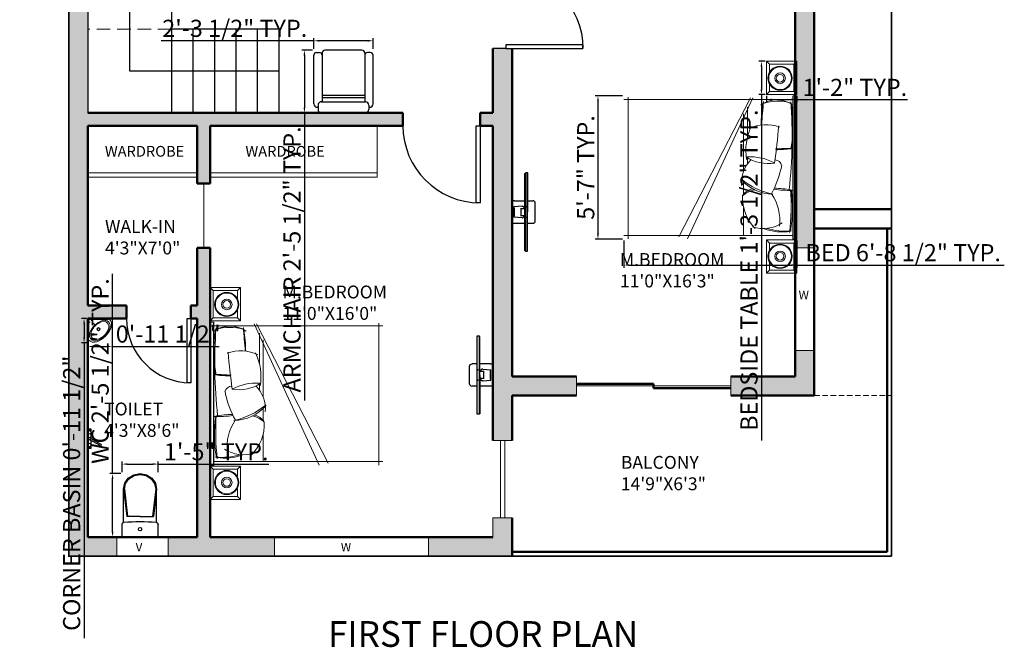
# Model space of a CAD drawing. Units: inches. Extents: x 3354 to 4308, y 1668 to 2317.
# Tile 9 of 11: x 3848 to 4308, y 1712 to 2005. Entities that reach past the tile are written whole.
import ezdxf

# ---------------------------------------------------------------- set-up
doc = ezdxf.new("R2010")
doc.units = ezdxf.units.IN
doc.linetypes.add('DASHED', pattern=[19.05, 12.7, -6.35])
for name, color, linetype, lineweight in [('0.10', 252, 'Continuous', 9), ('0.15', 34, 'Continuous', 15), ('A-ANNO-DIMS', 2, 'Continuous', 18), ('A-ANNO-TEXT', 7, 'Continuous', 18), ('A-AREA-IDEN', 3, 'Continuous', 18), ('A-DOOR', 3, 'Continuous', 25), ('A-FLOR-FIXT', 8, 'Continuous', 18), ('A-FLOR-OVHD', 8, 'DASHED', 18), ('A-FLOR-STRS', 7, 'Continuous', 25), ('A-FURN', 8, 'Continuous', 18), ('A-GLAZ', 4, 'Continuous', 18), ('A-WALL', 7, 'Continuous', 50), ('A-WALL-PATT', 8, 'Continuous', 13), ('C-PROP', 1, 'Continuous', 35)]:
    doc.layers.add(name, color=color, linetype=linetype, lineweight=lineweight)
for name, color, linetype in [('SANTEH', 7, 'Continuous'), ('window', 130, 'Continuous'), ('wood', 26, 'Continuous')]:
    doc.layers.add(name, color=color, linetype=linetype)
doc.styles.get("Standard").update_dxf_attribs({"font": 'arial.ttf'})
doc.dimstyles.new('ISO-25', dxfattribs={"dimtxt": 8, "dimasz": 2.5, "dimexe": 1.25, "dimexo": 0.625, "dimtad": 1, "dimdec": 1, "dimlunit": 3, "dimtxsty": 'Standard', "dimcen": 2.5, "dimadec": 0, "dimazin": 0, "dimtfac": 1, "dimtdec": 1, "dimtmove": 0, "dimatfit": 3, "dimfxl": 1, "dimarcsym": 0})

# ---------------------------------------------------------------- blocks, each defined once
blk = doc.blocks.new('*U3')
for p, q in [((0, 0), (0, -6)), ((36, 0), (36, -6))]:
    blk.add_line(p, q)
blk.add_lwpolyline([(0, 0), (0, 36), (1.75, 36), (1.75, 0)], close=True)
blk.add_arc((0, 0), 36, 0, 90)
blk = doc.blocks.new('A$C38B70996')
at = {"layer": 'wood'}
for p, q in [((0.06, 0.79), (0.06, 0.85)), ((0.11, 0.9), (0.74, 0.9)), ((0.79, 0.79), (0.79, 0.85)), ((0, 0.77), (0, 0.073)), ((0.06, 0.82), (0.05, 0.82)), ((0.74, 0.74), (0.11, 0.74)), ((0.12, 0.04), (0.12, 0.74)), ((0.73, 0.04), (0.73, 0.74)), ((0.79, 0.82), (0.8, 0.82)), ((0.85, 0.77), (0.85, 0.073)), ((0.73, 0.68), (0.12, 0.68)), ((0.73, 0.647), (0.12, 0.647)), ((0.04, 0.033), (0.08, 0.033)), ((0.16, 0), (0.69, 0)), ((0.81, 0.033), (0.77, 0.033))]:
    blk.add_line(p, q, dxfattribs=at)
for centre, radius, start, end in [((0.11, 0.85), 0.05, 90, 180), ((0.74, 0.85), 0.05, 0, 90), ((0.05, 0.77), 0.05, 90, 180), ((0.11, 0.79), 0.05, 180, 270), ((0.74, 0.79), 0.05, 270, 0), ((0.8, 0.77), 0.05, 360, 90), ((0.04, 0.073), 0.04, 180, 270), ((0.08, 0.073), 0.04, 270, 0), ((0.16, 0.04), 0.04, 180, 270), ((0.69, 0.04), 0.04, 270, 360), ((0.77, 0.073), 0.04, 180, 270), ((0.81, 0.073), 0.04, 270, 360)]:
    blk.add_arc(centre, radius, start, end, dxfattribs=at)
blk = doc.blocks.new('*U2')
for p, q in [((0, 0), (0, -6)), ((30, 0), (30, -6))]:
    blk.add_line(p, q)
blk.add_lwpolyline([(0, 0), (0, 30), (1.75, 30), (1.75, 0)], close=True)
blk.add_arc((0, 0), 30, 0, 90)
blk = doc.blocks.new('WC 2 Symb_109')
at = {"layer": 'SANTEH'}
for p, q in [((0, 0), (0, 380)), ((0, 380), (132, 380)), ((154, 365), (507, 365)), ((506, 365), (216, 331)), ((506, 356), (216, 322)), ((216, 190), (216, 331)), ((216, 190), (216, 49)), ((154, 15), (507, 15)), ((506, 24), (216, 58)), ((506, 15), (216, 49)), ((0, 0), (132, 0))]:
    blk.add_line(p, q, dxfattribs=at)
for points in [[(155, 360), (154, 364), (152, 368), (150, 371), (147, 374), (144, 377), (140, 379), (137, 380), (132, 380)], [(155, 20), (159, 62), (161, 105), (163, 147), (164, 190), (163, 233), (161, 275), (159, 318), (155, 360)], [(506, 24), (565, 37), (616, 73), (649, 126), (661, 190), (649, 254), (616, 307), (565, 343), (506, 356)], [(507, 15), (569, 28), (622, 66), (658, 123), (670, 190), (658, 257), (622, 314), (569, 352), (507, 365)], [(132, 0), (136, 0), (140, 1), (144, 3), (147, 6), (150, 9), (152, 12), (154, 16), (155, 20)]]:
    blk.add_lwpolyline(points, dxfattribs=at)
blk.add_lwpolyline([(84, 208), (70, 203), (65, 190), (70, 177), (84, 172), (97, 177), (102, 190), (97, 203)], close=True, dxfattribs=at)
blk = doc.blocks.new('Faucet - kit sink top')
at = {"layer": 'SANTEH'}
for p, q in [((-5.5, -0.75), (-5.5, -1.25)), ((-4.94278, -0.75), (-5.5, -0.75)), ((-5.5, -1.25), (-4.94278, -1.25)), ((-0.14775, -1.7441), (3.56698, -8.1782)), ((4.43301, -7.6782), (0.71828, -1.2441)), ((4.94278, -0.75), (5.5, -0.75)), ((5.5, -1.25), (4.94278, -1.25)), ((5.5, -0.75), (5.5, -1.25))]:
    blk.add_line(p, q, dxfattribs=at)
blk.add_lwpolyline([(-0.00587, -2), (-6, -2), (-6, 0), (6, 0), (6, -2), (1.15195, -2)], dxfattribs=at)
for centre, radius in [((-4, -1), 1), ((4, -1), 1), ((0, -1), 0.75)]:
    blk.add_circle(centre, radius, dxfattribs=at)
blk.add_arc((4, -7.9282), 0.5, 210, 30, dxfattribs=at)
blk = doc.blocks.new('s_11')
at = {"color": 0}
for p, q in [((-3, 6), (-3, 303)), ((-3, 6), (-3, 303)), ((-7, 252), (30, 252)), ((11, 19), (8, 238)), ((11, 234), (11, 270)), ((-6, 49), (30, 49)), ((12, 31), (12, 67)), ((237, 9), (18, 12)), ((30, 13), (66, 13)), ((48, -5), (48, 31)), ((233, 13), (269, 13)), ((251, -5), (251, 31)), ((302, -2), (4, -2)), ((302, -2), (4, -2))]:
    blk.add_line(p, q, dxfattribs=at)
at = {"color": 0, "extrusion": (0, 0, -1)}
for centre, major_axis, start_param, end_param in [((4, 303), (-5.13, 5.12), -0.785398, 0.025884), ((4, 303), (-5.13, 5.12), -0.785398, 0.025884), ((84, 219), (-87.2, 87.1), 0.025883, 1.117399), ((84, 219), (-87.2, 87.1), 0.025883, 1.117399), ((105, 236), (-61.5, 61.5), -1.180146, 1.180146), ((116, 223), (-56.4, 56.4), -1.140724, 1.140724), ((14, 15), (-239, 239), 1.117399, 2.024193), ((14, 15), (-239, 239), 1.117399, 2.024193), ((13, 14), (-232, 232), 1.180146, 1.961447), ((54, 55), (-183, 183), 1.140724, 2.000869), ((11, 252), (-5.13, 5.12), 3.141593, 9.424778), ((327, 329), (-232, 232), 4.321738, 5.10304), ((284, 285), (-183, 183), 4.282316, 5.142462), ((151, 152), (-16.4, 16.4), 3.141593, 9.424778), ((151, 152), (-10.3, 10.2), 3.141593, 9.424778), ((222, 118), (-56.4, 56.4), 2.000869, 4.282316), ((4, 6), (-5.13, 5.12), 3.926991, 5.497787), ((4, 6), (-5.13, 5.12), 3.926991, 5.497787), ((12, 49), (-5.13, 5.12), 3.141593, 9.424778), ((18, 19), (-5.13, 5.12), 3.939487, 5.485291), ((48, 13), (-5.13, 5.12), 3.141593, 9.424778), ((79, 80), (-8.98, 8.97), 3.141593, 9.424778), ((235, 107), (-61.5, 61.5), 1.961447, 4.321738), ((251, 13), (-5.13, 5.12), 3.141593, 9.424778), ((302, 6), (-5.13, 5.12), 3.115708, 3.926991), ((302, 6), (-5.13, 5.12), 3.115708, 3.926991), ((217, 86), (-87.2, 87.1), 2.024193, 3.11571), ((217, 86), (-87.2, 87.1), 2.024193, 3.11571)]:
    blk.add_ellipse(centre, major_axis=major_axis, ratio=0.999043, start_param=start_param, end_param=end_param, dxfattribs=at)
blk = doc.blocks.new('camita')
at = {"layer": '0.10'}
for p, q in [((-0.85, -0.045), (0.85, -0.045)), ((-0.805, -0.045), (-0.805, -2.048)), ((0.805, -0.045), (0.805, -2.048)), ((-0.827, -0.521), (0.846, -1.293)), ((-0.827, -0.548), (0.824, -1.399)), ((-0.716, -0.585), (-0.355, -0.585)), ((-0.638, -0.63), (0.043, -0.63)), ((-0.114, -0.585), (-0.049, -0.585)), ((0.175, -0.63), (0.318, -0.63)), ((0.474, -0.63), (0.805, -0.63)), ((-0.835, -2), (0.846, -2))]:
    blk.add_line(p, q, dxfattribs=at)
blk.add_lwpolyline([(-0.85, -0.041), (0.85, -0.041), (0.85, 0), (-0.85, 0)], close=True, dxfattribs=at)
for centre, radius, start, end in [((-0.457, -0.236), 0.344, 147.51, 213.8336), ((-0.2, -0.227), 0.586, 163.9263, 197.1409), ((-0.364, -5.846), 5.791, 83.8073, 94.1211), ((-0.51, -1.723), 1.678, 80.1255, 98.6619), ((2.353, -0.053), 2.58, 180.1063, 184.3854), ((-1.544, -0.245), 1.333, 359.9394, 7.5533), ((1.581, -0.289), 1.335, 170.3802, 178.9914), ((-1.44, -0.061), 1.712, 352.9291, 0.3959), ((0.452, -3.067), 3, 83.9026, 93.6759), ((0.486, -1.629), 1.578, 80.1602, 98.06), ((0.029, -0.138), 0.726, 342.5841, 6.0048), ((0.133, -0.17), 0.631, 339.923, 8.7433), ((-0.054, -0.363), 0.454, 159.3026, 206.5026), ((-1.33, -9.675), 9.499, 82.2708, 84.9399), ((-0.007, -0.258), 0.0828, 100.018, 179.736), ((-0.293, -1.438), 1.29, 61.9749, 77.8435), ((0.627, -0.752), 0.551, 82.9691, 124.6739), ((0.32, -0.394), 0.404, 341.4524, 33.4512), ((0.458, -0.545), 0.584, 151.0456, 184.1497), ((-0.534, -0.339), 0.487, 327.2644, 9.0473), ((-0.199, -0.274), 0.516, 310.7395, 359.0576), ((-0.567, -0.087), 0.906, 321.6953, 346.4626), ((-1.867, -14.986), 14.632, 84.6597, 85.7516), ((-0.46, 1.486), 1.909, 260.953, 268.6517), ((-0.2, 0.064), 0.667, 244.7809, 279.0606), ((0.179, -0.272), 0.383, 224.5284, 275.2229), ((0.438, -0.483), 0.19, 193.6849, 236.7035), ((0.571, -0.432), 0.315, 192.9388, 221.9636), ((0.361, -0.133), 0.51, 267.2589, 315.2997)]:
    blk.add_arc(centre, radius, start, end, dxfattribs=at)
blk = doc.blocks.new('VELADOR')
at = {"layer": '0.15'}
for p, q in [((-0.248, 0), (-0.203, -0.045)), ((0.248, 0), (0.202, -0.045)), ((-0.203, -0.405), (-0.248, -0.45)), ((0.248, -0.45), (0.202, -0.405))]:
    blk.add_line(p, q, dxfattribs=at)
blk.add_lwpolyline([(-0.248, 0), (-0.248, -0.45), (0.248, -0.45), (0.248, 0)], close=True, dxfattribs=at)
blk.add_lwpolyline([(0.092, -0.405), (0.202, -0.405), (0.202, -0.045), (-0.203, -0.045), (-0.203, -0.405), (-0.082, -0.405)], dxfattribs=at)
for radius in [0.18, 0.169, 0.0788, 0.0563]:
    blk.add_circle((0.005, -0.247), radius, dxfattribs=at)
blk = doc.blocks.new('TV')
at = {"color": 0}
for p, q in [((3967.27, 1784.85), (3967.05, 1784.65)), ((3967.76, 1763.68), (3967.54, 1763.86))]:
    blk.add_line(p, q, dxfattribs=at)
at = {"layer": 'window'}
for p, q in [((3967.54, 1763.86), (3967.05, 1784.65)), ((3966.53, 1775.82), (3964.33, 1775.61)), ((3964.34, 1775.34), (3964.45, 1775.34)), ((3964.34, 1775.31), (3964.43, 1775.32)), ((3964.41, 1777.23), (3967.22, 1777.3)), ((3966.14, 1775.2), (3967.01, 1775.22)), ((3966.14, 1775.18), (3967.27, 1775.2)), ((3966.14, 1775.18), (3966.14, 1775.2)), ((3966.3, 1773.29), (3966.26, 1775.18)), ((3968.01, 1777.32), (3969.36, 1777.35)), ((3964.39, 1773.06), (3964.48, 1773.06)), ((3964.39, 1773.04), (3964.5, 1773.04)), ((3966.61, 1772.66), (3964.4, 1772.77)), ((3966.19, 1773.28), (3967.31, 1773.31)), ((3966.19, 1773.26), (3967.05, 1773.28)), ((3966.19, 1773.26), (3966.19, 1773.28)), ((3964.55, 1771.15), (3967.36, 1771.22)), ((3968.15, 1771.24), (3969.5, 1771.27))]:
    blk.add_line(p, q, dxfattribs=at)
for points in [[(3968.33, 1763.69), (3967.83, 1784.86), (3967.27, 1784.85), (3967.76, 1763.68), (3968.33, 1763.69)], [(3963.86, 1771.81), (3963.75, 1776.54)], [(3964.4, 1772.77), (3964.33, 1775.61)], [(3964.48, 1773.06), (3964.43, 1775.32)], [(3964.5, 1773.04), (3964.45, 1775.34)], [(3970.16, 1771.96), (3970.05, 1776.69)]]:
    blk.add_lwpolyline(points, dxfattribs=at)
for points in [[(3966.53, 1775.82, -0.263666), (3966.93, 1775.69), (3967, 1775.57), (3967.01, 1775.22)], [(3966.61, 1772.66, 0.263666), (3967, 1772.81), (3967.06, 1772.93), (3967.05, 1773.28)]]:
    blk.add_lwpolyline(points, format="xyb", dxfattribs=at)
for centre, radius in [((3963.91, 1775.73), 0.0679), ((3963.93, 1775.17), 0.0679), ((3967.77, 1775.68), 0.0451), ((3963.94, 1774.6), 0.0679), ((3963.95, 1774.04), 0.0679), ((3963.97, 1773.48), 0.0679), ((3963.98, 1772.92), 0.0679), ((3963.99, 1772.35), 0.0679), ((3967.83, 1772.86), 0.0451), ((3964.01, 1771.79), 0.0679)]:
    blk.add_circle(centre, radius, dxfattribs=at)
for centre, start, end in [((3964.42, 1776.56), 91.3414, 181.3414), ((3969.38, 1776.67), 1.3414, 91.3414), ((3964.53, 1771.83), 181.3414, 271.3414), ((3969.49, 1771.94), 271.3414, 1.3414)]:
    blk.add_arc(centre, 0.676, start, end, dxfattribs=at)
blk = doc.blocks.new('*D54')
at = {"layer": 'A-ANNO-DIMS', "color": 0, "lineweight": -2, "transparency": 16777216}
for p, q in [((3985.11, 1990.57), (3980.1, 1990.57)), ((3981.35, 1988.07), (3981.35, 1963.8)), ((3985.11, 1961.3), (3980.1, 1961.3)), ((3981.35, 1961.3), (3981.35, 1826.97))]:
    blk.add_line(p, q, dxfattribs=at)
at = {"layer": 'A-ANNO-DIMS', "color": 0, "transparency": 16777216}
for points in [[(3980.93, 1988.07), (3981.76, 1988.07), (3981.35, 1990.57)], [(3980.93, 1963.8), (3981.76, 1963.8), (3981.35, 1961.3)]]:
    blk.add_solid(points, dxfattribs=at)
at = {"layer": 'Defpoints', "color": 0, "transparency": 16777216}
for p in [(3985.74, 1990.57), (3981.35, 1961.3), (3985.74, 1961.3)]:
    blk.add_point(p, dxfattribs=at)
at = {"layer": 'A-ANNO-DIMS', "color": 0, "transparency": 16777216, "insert": (3976.58, 1892.88), "char_height": 8, "attachment_point": 5, "rotation": 90}
blk.add_mtext('ARMCHAIR 2\'-5 1/2" TYP.', dxfattribs=at)
blk = doc.blocks.new('*D55')
at = {"layer": 'A-ANNO-DIMS', "color": 0, "lineweight": -2, "transparency": 16777216}
for p, q in [((3985.74, 1994.97), (3914.45, 1994.97)), ((3985.74, 1991.2), (3985.74, 1996.22)), ((4010.89, 1994.97), (3988.24, 1994.97)), ((4013.39, 1991.2), (4013.39, 1996.22))]:
    blk.add_line(p, q, dxfattribs=at)
at = {"layer": 'A-ANNO-DIMS', "color": 0, "transparency": 16777216}
for points in [[(3988.24, 1995.38), (3988.24, 1994.55), (3985.74, 1994.97)], [(4010.89, 1995.38), (4010.89, 1994.55), (4013.39, 1994.97)]]:
    blk.add_solid(points, dxfattribs=at)
at = {"layer": 'Defpoints', "color": 0, "transparency": 16777216}
for p in [(3985.74, 1994.97), (3985.74, 1990.57), (4013.39, 1990.57)]:
    blk.add_point(p, dxfattribs=at)
at = {"layer": 'A-ANNO-DIMS', "color": 0, "transparency": 16777216, "insert": (3948.84, 1999.73), "char_height": 8, "attachment_point": 5}
blk.add_mtext('2\'-3 1/2" TYP.', dxfattribs=at)
blk = doc.blocks.new('*D60')
at = {"layer": 'A-ANNO-DIMS', "color": 0, "lineweight": -2, "transparency": 16777216}
for p, q in [((3891.8, 1792.9), (3891.8, 1886.11)), ((3895.62, 1792.9), (3890.55, 1792.9)), ((3891.8, 1765.8), (3891.8, 1790.4)), ((3895.62, 1763.3), (3890.55, 1763.3))]:
    blk.add_line(p, q, dxfattribs=at)
at = {"layer": 'A-ANNO-DIMS', "color": 0, "transparency": 16777216}
for points in [[(3891.39, 1790.4), (3892.22, 1790.4), (3891.8, 1792.9)], [(3891.39, 1765.8), (3892.22, 1765.8), (3891.8, 1763.3)]]:
    blk.add_solid(points, dxfattribs=at)
at = {"layer": 'Defpoints', "color": 0, "transparency": 16777216}
for p in [(3891.8, 1792.9), (3896.24, 1792.9), (3896.24, 1763.3)]:
    blk.add_point(p, dxfattribs=at)
at = {"layer": 'A-ANNO-DIMS', "color": 0, "transparency": 16777216, "insert": (3887.04, 1840.76), "char_height": 8, "attachment_point": 5, "rotation": 90}
blk.add_mtext('WC 2\'-5 1/2" TYP.', dxfattribs=at)
blk = doc.blocks.new('*D61')
at = {"layer": 'A-ANNO-DIMS', "color": 0, "lineweight": -2, "transparency": 16777216}
for p, q in [((3896.24, 1793.53), (3896.24, 1798.59)), ((3898.74, 1797.34), (3910.53, 1797.34)), ((3913.03, 1793.53), (3913.03, 1798.59)), ((3913.03, 1797.34), (3964.8, 1797.34))]:
    blk.add_line(p, q, dxfattribs=at)
at = {"layer": 'A-ANNO-DIMS', "color": 0, "transparency": 16777216}
for points in [[(3898.74, 1797.76), (3898.74, 1796.93), (3896.24, 1797.34)], [(3910.53, 1797.76), (3910.53, 1796.93), (3913.03, 1797.34)]]:
    blk.add_solid(points, dxfattribs=at)
at = {"layer": 'Defpoints', "color": 0, "transparency": 16777216}
for p in [(3913.03, 1797.34), (3896.24, 1792.9), (3913.03, 1792.9)]:
    blk.add_point(p, dxfattribs=at)
at = {"layer": 'A-ANNO-DIMS', "color": 0, "transparency": 16777216, "insert": (3940.17, 1802.05), "char_height": 8, "attachment_point": 5}
blk.add_mtext('1\'-5" TYP.', dxfattribs=at)
blk = doc.blocks.new('*D62')
at = {"layer": 'A-ANNO-DIMS', "color": 0, "lineweight": -2, "transparency": 16777216}
for p, q in [((4196.37, 1985.4), (4193.41, 1985.4)), ((4194.66, 1982.9), (4194.66, 1972.35)), ((4196.37, 1969.85), (4193.41, 1969.85)), ((4194.66, 1969.85), (4194.66, 1808.37))]:
    blk.add_line(p, q, dxfattribs=at)
at = {"layer": 'A-ANNO-DIMS', "color": 0, "transparency": 16777216}
for points in [[(4194.25, 1982.9), (4195.08, 1982.9), (4194.66, 1985.4)], [(4194.25, 1972.35), (4195.08, 1972.35), (4194.66, 1969.85)]]:
    blk.add_solid(points, dxfattribs=at)
at = {"layer": 'Defpoints', "color": 0, "transparency": 16777216}
for p in [(4196.99, 1985.4), (4194.66, 1969.85), (4196.99, 1969.85)]:
    blk.add_point(p, dxfattribs=at)
at = {"layer": 'A-ANNO-DIMS', "color": 0, "transparency": 16777216, "insert": (4189.9, 1887.86), "char_height": 8, "attachment_point": 5, "rotation": 90}
blk.add_mtext('BEDSIDE TABLE 1\'-3 1/2" TYP.', dxfattribs=at)
blk = doc.blocks.new('*D63')
at = {"layer": 'A-ANNO-DIMS', "color": 0, "lineweight": -2, "transparency": 16777216}
for p, q in [((4196.99, 1969.23), (4196.99, 1966.27)), ((4199.49, 1967.52), (4208.63, 1967.52)), ((4211.13, 1969.23), (4211.13, 1966.27)), ((4211.13, 1967.52), (4262.89, 1967.52))]:
    blk.add_line(p, q, dxfattribs=at)
at = {"layer": 'A-ANNO-DIMS', "color": 0, "transparency": 16777216}
for points in [[(4199.49, 1967.94), (4199.49, 1967.1), (4196.99, 1967.52)], [(4208.63, 1967.94), (4208.63, 1967.1), (4211.13, 1967.52)]]:
    blk.add_solid(points, dxfattribs=at)
at = {"layer": 'Defpoints', "color": 0, "transparency": 16777216}
for p in [(4196.99, 1969.85), (4211.13, 1969.85), (4211.13, 1967.52)]:
    blk.add_point(p, dxfattribs=at)
at = {"layer": 'A-ANNO-DIMS', "color": 0, "transparency": 16777216, "insert": (4238.26, 1972.16), "char_height": 8, "attachment_point": 5}
blk.add_mtext('1\'-2" TYP.', dxfattribs=at)
blk = doc.blocks.new('*D64')
at = {"layer": 'A-ANNO-DIMS', "color": 0, "lineweight": -2, "transparency": 16777216}
for p, q in [((4130.47, 1901.7), (4130.47, 1888.98)), ((4211.13, 1901.7), (4211.13, 1888.98)), ((4132.97, 1890.23), (4208.63, 1890.23)), ((4211.13, 1890.23), (4308.02, 1890.23))]:
    blk.add_line(p, q, dxfattribs=at)
at = {"layer": 'A-ANNO-DIMS', "color": 0, "transparency": 16777216}
for points in [[(4132.97, 1890.65), (4132.97, 1889.81), (4130.47, 1890.23)], [(4208.63, 1890.65), (4208.63, 1889.81), (4211.13, 1890.23)]]:
    blk.add_solid(points, dxfattribs=at)
at = {"layer": 'Defpoints', "color": 0, "transparency": 16777216}
for p in [(4130.47, 1902.33), (4211.13, 1902.33), (4211.13, 1890.23)]:
    blk.add_point(p, dxfattribs=at)
at = {"layer": 'A-ANNO-DIMS', "color": 0, "transparency": 16777216, "insert": (4260.82, 1894.99), "char_height": 8, "attachment_point": 5}
blk.add_mtext('BED 6\'-8 1/2" TYP.', dxfattribs=at)
blk = doc.blocks.new('*D65')
at = {"layer": 'A-ANNO-DIMS', "color": 0, "lineweight": -2, "transparency": 16777216}
for p, q in [((4129.85, 1969.27), (4117.12, 1969.27)), ((4118.37, 1966.77), (4118.37, 1904.83)), ((4129.85, 1902.33), (4117.12, 1902.33))]:
    blk.add_line(p, q, dxfattribs=at)
at = {"layer": 'A-ANNO-DIMS', "color": 0, "transparency": 16777216}
for points in [[(4117.96, 1966.77), (4118.79, 1966.77), (4118.37, 1969.27)], [(4117.96, 1904.83), (4118.79, 1904.83), (4118.37, 1902.33)]]:
    blk.add_solid(points, dxfattribs=at)
at = {"layer": 'Defpoints', "color": 0, "transparency": 16777216}
for p in [(4130.47, 1969.27), (4118.37, 1902.33), (4130.47, 1902.33)]:
    blk.add_point(p, dxfattribs=at)
at = {"layer": 'A-ANNO-DIMS', "color": 0, "transparency": 16777216, "insert": (4113.68, 1935.8), "char_height": 8, "attachment_point": 5, "rotation": 90}
blk.add_mtext('5\'-7" TYP.', dxfattribs=at)
blk = doc.blocks.new('*D94')
at = {"layer": 'A-ANNO-DIMS', "color": 0, "lineweight": -2, "transparency": 16777216}
for p, q in [((3879.59, 1865.37), (3877.26, 1865.37)), ((3878.51, 1862.87), (3878.51, 1856.47)), ((3879.59, 1853.97), (3877.26, 1853.97)), ((3878.51, 1853.97), (3878.51, 1716.01))]:
    blk.add_line(p, q, dxfattribs=at)
at = {"layer": 'A-ANNO-DIMS', "color": 0, "transparency": 16777216}
for points in [[(3878.09, 1862.87), (3878.92, 1862.87), (3878.51, 1865.37)], [(3878.09, 1856.47), (3878.92, 1856.47), (3878.51, 1853.97)]]:
    blk.add_solid(points, dxfattribs=at)
at = {"layer": 'Defpoints', "color": 0, "transparency": 16777216}
for p in [(3880.22, 1865.37), (3878.51, 1853.97), (3880.22, 1853.97)]:
    blk.add_point(p, dxfattribs=at)
at = {"layer": 'A-ANNO-DIMS', "color": 0, "transparency": 16777216, "insert": (3873.74, 1783.74), "char_height": 8, "attachment_point": 5, "rotation": 90}
blk.add_mtext('CORNER BASIN 0\'-11 1/2"', dxfattribs=at)
blk = doc.blocks.new('*D95')
at = {"layer": 'A-ANNO-DIMS', "color": 0, "lineweight": -2, "transparency": 16777216}
for p, q in [((3880.22, 1853.34), (3880.22, 1851.01)), ((3882.72, 1852.26), (3889.11, 1852.26)), ((3891.61, 1853.34), (3891.61, 1851.01)), ((3891.61, 1852.26), (3941.49, 1852.26))]:
    blk.add_line(p, q, dxfattribs=at)
at = {"layer": 'A-ANNO-DIMS', "color": 0, "transparency": 16777216}
for points in [[(3882.72, 1852.67), (3882.72, 1851.84), (3880.22, 1852.26)], [(3889.11, 1852.67), (3889.11, 1851.84), (3891.61, 1852.26)]]:
    blk.add_solid(points, dxfattribs=at)
at = {"layer": 'Defpoints', "color": 0, "transparency": 16777216}
for p in [(3880.22, 1853.97), (3891.61, 1853.97), (3891.61, 1852.26)]:
    blk.add_point(p, dxfattribs=at)
at = {"layer": 'A-ANNO-DIMS', "color": 0, "transparency": 16777216, "insert": (3917.8, 1857.02), "char_height": 8, "attachment_point": 5}
blk.add_mtext('0\'-11 1/2"', dxfattribs=at)

msp = doc.modelspace()

# ---------------------------------------------------------------- hatches: boundary and pattern name
at = {"layer": 'A-WALL-PATT', "transparency": 33554687}
h = msp.add_hatch(color=256, dxfattribs=at)
h.dxf.hatch_style = 1
h.paths.add_polyline_path([(4078.33, 1991.3), (4069.33, 1991.3), (4069.33, 1961.3), (4063.33, 1961.3), (4063.33, 1955.3), (4069.33, 1955.3), (4069.33, 1808.3), (4078.33, 1808.3), (4078.33, 1829.3), (4108.33, 1829.3), (4108.33, 1838.3), (4078.33, 1838.3)])
h.paths.add_polyline_path([(4219.33, 1850.3), (4210.33, 1850.3), (4210.33, 1838.3), (4180.33, 1838.3), (4180.33, 1829.3), (4219.33, 1829.3)])
h.paths.add_polyline_path([(4219.33, 2075.3), (4210.33, 2075.3), (4210.33, 2039.3), (4206.56, 2039.3), (4138.33, 2039.3), (4138.33, 2042.3), (4132.33, 2042.3), (4132.33, 2009.3), (4138.33, 2009.3), (4138.33, 2033.3), (4210.33, 2033.3), (4210.33, 1985.4), (4211.13, 1985.4), (4211.13, 1969.85), (4211.13, 1902.33), (4211.13, 1898.3), (4219.33, 1898.3)])
h.paths.add_polyline_path([(4078.33, 2111.3), (4132.33, 2111.3), (4132.33, 2072.3), (4138.33, 2072.3), (4138.33, 2111.3), (4210.33, 2111.3), (4210.33, 2099.3), (4219.33, 2099.3), (4219.33, 2150.3), (4210.33, 2150.3), (4210.33, 2117.3), (4078.33, 2117.3), (4078.33, 2249.3), (4108.33, 2249.3), (4108.33, 2258.3), (4030.33, 2258.3), (4030.33, 2249.3), (4072.33, 2249.3), (4072.33, 2117.3), (4069.33, 2117.3), (4069.33, 2111.3), (4069.33, 2027.3), (4075.33, 2027.3), (4078.33, 2027.3), (4078.33, 2033.3), (4102.33, 2033.3), (4102.33, 2039.3), (4078.33, 2039.3)])
h.paths.add_polyline_path([(4219.33, 2258.3), (4180.33, 2258.3), (4180.33, 2249.3), (4210.33, 2249.3), (4210.33, 2210.3), (4219.33, 2210.3)], flags=17)
h.paths.add_polyline_path([(3970.33, 2258.3), (3919.33, 2258.3), (3919.33, 2249.3), (3922.3, 2249.3), (3934.33, 2249.3), (3934.33, 2159.3), (3940.33, 2159.3), (3940.33, 2249.3), (3970.33, 2249.3)], flags=17)
h.paths.add_polyline_path([(3880.33, 2111.3), (4033.33, 2111.3), (4033.33, 2117.3), (3940.33, 2117.3), (3940.33, 2129.3), (3934.33, 2129.3), (3934.33, 2117.3), (3880.33, 2117.3), (3880.33, 2159.3), (3901.33, 2159.3), (3901.33, 2165.3), (3880.33, 2165.3), (3880.33, 2249.3), (3895.33, 2249.3), (3895.33, 2258.3), (3871.33, 2258.3), (3871.33, 1754.3), (3893.83, 1754.3), (3893.83, 1763.3), (3880.33, 1763.3), (3880.33, 1865.3), (3898.33, 1865.3), (3898.33, 1871.3), (3880.33, 1871.3), (3880.33, 1955.3), (3931.33, 1955.3), (3931.33, 1928.3), (3937.33, 1928.3), (3937.33, 1955.3), (4027.33, 1955.3), (4027.33, 1961.3), (3880.33, 1961.3)])
h.paths.add_polyline_path([(3967.33, 1763.3), (3937.33, 1763.3), (3937.33, 1898.3), (3931.33, 1898.3), (3931.33, 1871.3), (3928.33, 1871.3), (3928.33, 1865.3), (3931.33, 1865.3), (3931.33, 1763.3), (3917.83, 1763.3), (3917.83, 1754.3), (3967.33, 1754.3)], flags=17)
h.paths.add_polyline_path([(4078.33, 1772.3), (4069.33, 1772.3), (4069.33, 1763.3), (4039.33, 1763.3), (4039.33, 1754.3), (4078.33, 1754.3)])

# ---------------------------------------------------------------- linework, layer by layer
at = {"layer": 'A-FLOR-OVHD', "ltscale": 0.5}
msp.add_line((3919.33, 2000.3), (3880.33, 2000.3), dxfattribs=at)
at = {"layer": 'A-FLOR-OVHD', "ltscale": 0.2}
msp.add_line((4219.33, 1829.3), (4255.33, 1829.3), dxfattribs=at)
at = {"layer": 'A-FLOR-STRS'}
for p, q in [((3880.33, 2111.3), (3880.33, 1961.3)), ((3919.33, 2072.3), (3919.33, 1961.3)), ((3969.33, 2000.3), (3919.33, 2000.3)), ((3929.33, 2000.3), (3929.33, 1961.3)), ((3939.33, 2000.3), (3939.33, 1961.3)), ((3949.33, 2000.3), (3949.33, 1961.3)), ((3959.33, 2000.3), (3959.33, 1961.3)), ((3969.33, 2000.3), (3969.33, 1961.3))]:
    msp.add_line(p, q, dxfattribs=at)
msp.add_lwpolyline([(3969.33, 1980.8), (3899.83, 1980.8), (3899.83, 2091.8), (3963.6, 2091.8)], dxfattribs=at)
at = {"layer": 'A-FURN'}
for p, q in [((4015.33, 1955.3), (4015.33, 1931.3)), ((4015.33, 1933.3), (3937.33, 1933.3)), ((4015.33, 1931.3), (3937.33, 1931.3)), ((3934.33, 1928.3), (3934.33, 1898.3))]:
    msp.add_line(p, q, dxfattribs=at)
at = {"layer": 'A-GLAZ'}
for p, q in [((4078.33, 1991.3), (4069.33, 1991.3)), ((3931.33, 1933.3), (3880.33, 1933.3)), ((3931.33, 1931.3), (3880.33, 1931.3)), ((4210.33, 1898.3), (4219.33, 1898.3)), ((4210.33, 1850.3), (4219.33, 1850.3)), ((4108.33, 1838.3), (4108.33, 1829.3)), ((4180.33, 1838.3), (4180.33, 1829.3)), ((4108.33, 1833.8), (4180.33, 1833.8)), ((4069.33, 1808.3), (4078.33, 1808.3)), ((4072.83, 1808.3), (4072.83, 1772.3)), ((4074.83, 1808.3), (4074.83, 1772.3)), ((4069.33, 1772.3), (4078.33, 1772.3)), ((4069.33, 1772.3), (4069.33, 1763.3)), ((3893.83, 1763.3), (3893.83, 1754.3)), ((3917.83, 1763.3), (3917.83, 1754.3)), ((3967.33, 1763.3), (3967.33, 1754.3)), ((4039.33, 1763.3), (4039.33, 1754.3))]:
    msp.add_line(p, q, dxfattribs=at)
at = {"layer": 'A-WALL'}
for p, q in [((4219.33, 1829.3), (4219.33, 2258.3)), ((4210.33, 1838.3), (4210.33, 2033.3)), ((4069.33, 1991.3), (4069.33, 1961.3)), ((4078.33, 1991.3), (4078.33, 1838.3)), ((4027.33, 1961.3), (3880.33, 1961.3)), ((4027.33, 1961.3), (4027.33, 1955.3)), ((4069.33, 1961.3), (4063.33, 1961.3)), ((4063.33, 1961.3), (4063.33, 1955.3)), ((3880.33, 1955.3), (3880.33, 1871.3)), ((3931.33, 1955.3), (3880.33, 1955.3)), ((3931.33, 1955.3), (3931.33, 1928.3)), ((4027.33, 1955.3), (3937.33, 1955.3)), ((3937.33, 1955.3), (3937.33, 1928.3)), ((4069.33, 1955.3), (4063.33, 1955.3)), ((4069.33, 1955.3), (4069.33, 1808.3)), ((3937.33, 1928.3), (3931.33, 1928.3)), ((4219.33, 1916.3), (4255.33, 1916.3)), ((4219.33, 1907.3), (4255.33, 1907.3)), ((4253.33, 1756.3), (4253.33, 1907.3)), ((3937.33, 1898.3), (3931.33, 1898.3)), ((3931.33, 1898.3), (3931.33, 1871.3)), ((3937.33, 1898.3), (3937.33, 1763.3)), ((3880.33, 1871.3), (3898.33, 1871.3)), ((3898.33, 1871.3), (3898.33, 1865.3)), ((3928.33, 1871.3), (3931.33, 1871.3)), ((3928.33, 1871.3), (3928.33, 1865.3)), ((3880.33, 1865.3), (3898.33, 1865.3)), ((3880.33, 1865.3), (3880.33, 1763.3)), ((3928.33, 1865.3), (3931.33, 1865.3)), ((3931.33, 1865.3), (3931.33, 1763.3)), ((4078.33, 1838.3), (4108.33, 1838.3)), ((4180.33, 1838.3), (4210.33, 1838.3)), ((4144.33, 1834.8), (4108.33, 1834.8)), ((4144.33, 1833.8), (4144.33, 1834.8)), ((4144.33, 1833.8), (4144.33, 1832.8)), ((4078.33, 1829.3), (4108.33, 1829.3)), ((4078.33, 1829.3), (4078.33, 1808.3)), ((4144.33, 1832.8), (4180.33, 1832.8)), ((4180.33, 1829.3), (4219.33, 1829.3)), ((4078.33, 1772.3), (4078.33, 1754.3)), ((3880.33, 1763.3), (3931.33, 1763.3)), ((3937.33, 1763.3), (4069.33, 1763.3)), ((4078.33, 1756.3), (4253.33, 1756.3))]:
    msp.add_line(p, q, dxfattribs=at)
at = {"layer": 'C-PROP'}
msp.add_lwpolyline([(4255.33, 1754.3), (4255.33, 2294.3), (3871.33, 2294.3), (3871.33, 1754.3), (4255.33, 1754.3)], dxfattribs=at)

# ---------------------------------------------------------------- block references
at = {"layer": 'A-DOOR', "xscale": -1, "rotation": 270}
msp.add_blockref('*U3', (4075.33, 1991.3), dxfattribs=at)
at = {"layer": 'A-DOOR', "rotation": 180}
for name, p in [('*U3', (4063.33, 1955.3)), ('*U2', (3928.33, 1865.3))]:
    msp.add_blockref(name, p, dxfattribs=at)
at = {"layer": 'A-FLOR-FIXT'}
for name, p, xscale, yscale, zscale, rotation in [('s_11', (3880.38, 1865.15), 0.0320644972991817, 0.0320644972991817, 0.0320644972991817, 270), ('Faucet - kit sink top', (3880.33, 1809.23), -0.7356136897818673, 0.7356136897818673, 0.7356136897818673, 90), ('WC 2 Symb_109', (3896.24, 1763.3), -0.0441898926459964, 0.0441898926459964, 0.0441898926459964, 270.0000000000001)]:
    msp.add_blockref(name, p, dxfattribs=dict(at, xscale=xscale, yscale=yscale, zscale=zscale, rotation=rotation))
at = {"layer": 'A-FURN'}
for name, p, xscale, yscale, zscale, rotation in [('A$C38B70996', (4013.39, 1990.57), 32.53084308163255, 32.53084308163255, 32.53084308163255, 180), ('VELADOR', (4211.13, 1977.63), 31.41542173157097, 31.41542173157097, 31.41542173157097, 270), ('camita', (4211.13, 1935.8), 39.375, 39.375, 39.375, 270), ('TV', (-2832.92, -969.73), 1.724488909621177, 1.724488909621177, 1.724488909621177, 358.5430845181614), ('VELADOR', (4211.13, 1894.18), -31.41542173157097, 31.41542173157097, 31.41542173157097, 269.9999999999999), ('VELADOR', (3937.33, 1872.03), -31.41542173157097, 31.41542173157097, 31.41542173157097, 90), ('camita', (3937.33, 1830.2), -39.375, 39.375, 39.375, 90), ('TV', (10980.44, -1045.86), -1.724488909621177, 1.724488909621177, 1.724488909621177, 1.456915481838603), ('VELADOR', (3937.33, 1788.58), 31.41542173157097, 31.41542173157097, 31.41542173157097, 90.00000000000011)]:
    msp.add_blockref(name, p, dxfattribs=dict(at, xscale=xscale, yscale=yscale, zscale=zscale, rotation=rotation))

# ---------------------------------------------------------------- texts
at = {"layer": 'A-ANNO-TEXT', "attachment_point": 1}
for s, width, insert, char_height in [('WARDROBE', 74.5832, (3888.21, 1945.85), 5), ('WARDROBE', 74.5832, (3953.8, 1945.85), 5), ('\\pxt6;{W}', 32.7844, (4212.02, 1878.24), 4), ('\\pxt6;{V}', 32.7844, (3902.57, 1760.57), 4), ('\\pxt6;{W}', 32.7844, (3998.36, 1760.57), 4), ('FIRST FLOOR PLAN', 202.1172, (3992.36, 1724.02), 12)]:
    msp.add_mtext_dynamic_manual_height_columns(s, width=width, gutter_width=12.5, heights=[0], dxfattribs=dict(at, insert=insert, char_height=char_height))
at = {"layer": 'A-AREA-IDEN', "char_height": 6, "attachment_point": 1}
for s, insert in [('WALK-IN\\P4\'3"X7\'0"', (3888.29, 1911.22)), ('M.BEDROOM\\P11\'0"X16\'3"', (4128.61, 1895.82)), ('M.BEDROOM\\P11\'0"X16\'0"', (3971.14, 1880.68)), ('TOILET\\P4\'3"X8\'6"', (3887.87, 1826.06)), ('BALCONY\\P14\'9"X6\'3"', (4129.04, 1801.14))]:
    msp.add_mtext_dynamic_manual_height_columns(s, width=74.5832, gutter_width=12.5, heights=[0], dxfattribs=dict(at, insert=insert))

# ---------------------------------------------------------------- dimensions: what is measured, and where the dimension line sits
at = {"layer": 'A-ANNO-DIMS'}
for base, p1, p2, angle, text, picture, middle in [((3985.7374, 1994.9659), (4013.3886, 1990.5742), (3985.7374, 1990.5742), 180, '<> TYP.', '*D55', (3948.8416, 1999.7301)), ((3981.35, 1961.3), (3985.74, 1990.57), (3985.74, 1961.3), 270, 'ARMCHAIR <> TYP.', '*D54', (3976.58, 1892.88)), ((4194.6621, 1969.8524), (4196.9947, 1985.403), (4196.9947, 1969.8524), 270, 'BEDSIDE TABLE <> TYP.', '*D62', (4189.8979, 1887.8625)), ((4118.37, 1902.33), (4130.47, 1969.27), (4130.47, 1902.33), 270, '<> TYP.', '*D65', (4113.68, 1935.8)), ((3891.8, 1792.9), (3896.24, 1763.3), (3896.24, 1792.9), 90, 'WC <> TYP.', '*D60', (3887.04, 1840.76)), ((3878.51, 1853.97), (3880.22, 1865.37), (3880.22, 1853.97), 270, 'CORNER BASIN <>', '*D94', (3873.74, 1783.74)), ((3913.03, 1797.34), (3896.24, 1792.9), (3913.03, 1792.9), 0, '<> TYP.', '*D61', (3940.17, 1802.05))]:
    dim = msp.add_linear_dim(base=base, p1=p1, p2=p2, angle=angle, text=text, dimstyle='ISO-25', override={"dimdec": 1, "dimrnd": 0, "dimzin": 1, "dimlunit": 4, "dimfrac": 2}, dxfattribs=at)
    dim.commit()
    dim.dimension.update_dxf_attribs({"geometry": picture, "text_midpoint": middle})
for base, p1, p2, text, picture, middle in [((4211.13, 1967.52), (4196.99, 1969.85), (4211.13, 1969.85), '<> TYP.', '*D63', (4238.26, 1972.16)), ((4211.13, 1890.23), (4130.47, 1902.33), (4211.13, 1902.33), 'BED <> TYP.', '*D64', (4260.82, 1894.99))]:
    dim = msp.add_linear_dim(base=base, p1=p1, p2=p2, text=text, dimstyle='ISO-25', override={"dimdec": 1, "dimrnd": 0, "dimzin": 1, "dimlunit": 4, "dimfrac": 2}, dxfattribs=at)
    dim.commit()
    dim.dimension.update_dxf_attribs({"geometry": picture, "text_midpoint": middle})
dim = msp.add_linear_dim(base=(3891.61, 1852.26), p1=(3880.22, 1853.97), p2=(3891.61, 1853.97), dimstyle='ISO-25', override={"dimdec": 1, "dimrnd": 0, "dimzin": 1, "dimlunit": 4, "dimfrac": 2}, dxfattribs=at)
dim.commit()
dim.dimension.update_dxf_attribs({"geometry": '*D95', "text_midpoint": (3917.8, 1857.02)})

doc.saveas('drawing.dxf')
